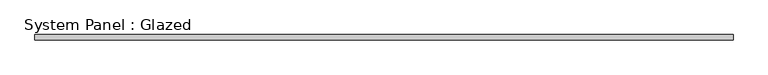
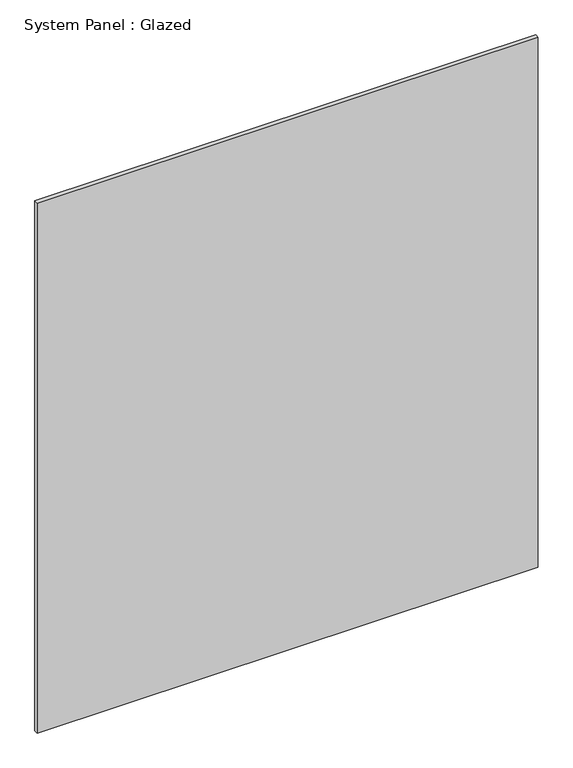
"""IFC4 building model written with IfcOpenShell, lengths in millimetres: plate geometry, System Panel : Glazed."""

from ifc_helpers import new_model, si_unit, origin, origin_with_axes, place, context, project, spatial, polyline, outline, extrude, source, transform, mapped, element, save


def system_panel_glazed_b9555dd7(model_context):
    return source(origin(), model_context, "Body", "SweptSolid", [
        extrude(outline(polyline([(1715.9253139, 19.05), (-1715.9253139, 19.05), (-1715.9253139, 44.45), (1715.9253139, 44.45), (1715.9253139, 19.05)])), origin_with_axes(), (0.0, 0.0, 1.0), 3835.4),
    ])


if __name__ == "__main__":
    model = new_model("IFC4")
    model_context = context("Model", 3, world=origin())
    ifc_project = project(units=[si_unit("LENGTHUNIT", "METRE", prefix="MILLI")], contexts=[model_context])
    site = spatial("IfcSite", under=ifc_project)
    building = spatial("IfcBuilding", under=site)
    placement = place(None, origin())
    system_panel_glazed_shape = system_panel_glazed_b9555dd7(model_context)
    element("IfcPlate", 1, ObjectType="System Panel : Glazed", at=placement, inside=building, context=model_context, shape_type="MappedRepresentation", body=[
        mapped(system_panel_glazed_shape, transform((0.0, 0.0, 0.0), x_axis=(1.0, 0.0, 0.0), y_axis=(0.0, 1.0, 0.0), z_axis=(0.0, 0.0, 1.0))),
    ])
    save(model, "model.ifc")

# Revit data of these elements
# Type "System Panel : Glazed"
#   Construction Type Id = "GSP4R"
#   Analytic Construction = "1/8 in Pilkington single glazing"
#   Visual Light Transmittance = 0.9
#   Solar Heat Gain Coefficient = 0.86
#   Heat Transfer Coefficient (U) = 1.18115 BTU/(h·ft²·°F)
# Element 1 (IfcPlate, "System Panel : Glazed")
#   Materials on its faces: "Glass"
# Materials
#   "Glass": class "Glass", colour RGB 0 128 192, transparency 0.75, Description = "Soda Lime Glass", Cost = 0
